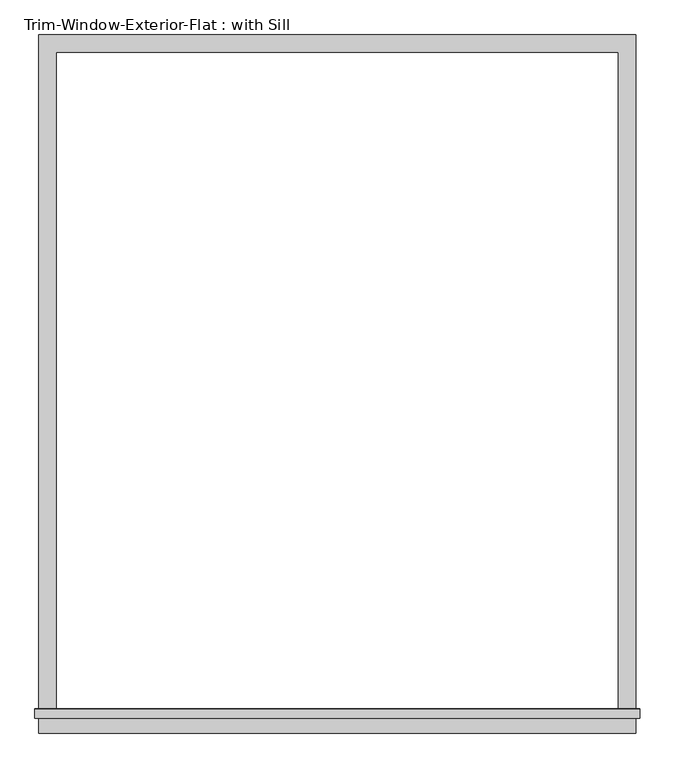
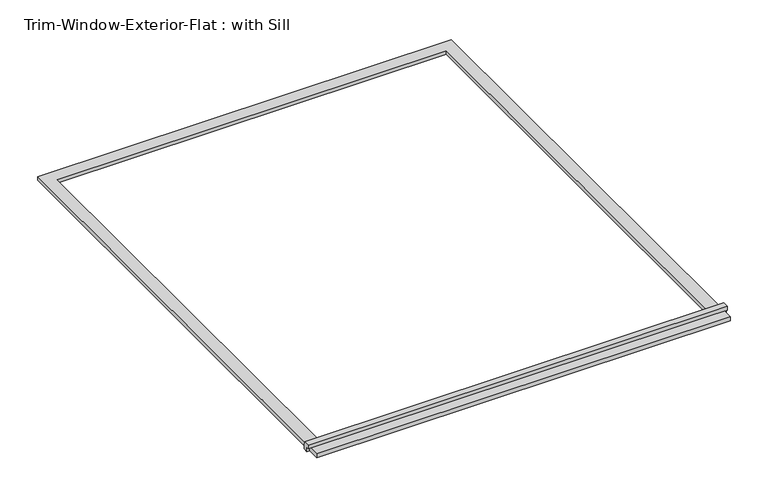
"""IFC4 building model written with IfcOpenShell, lengths in millimetres: proxy geometry, Trim-Window-Exterior-Flat : with Sill."""

from ifc_helpers import new_model, si_unit, frame, origin, origin_with_axes, place, context, project, spatial, polyline, outline, extrude, source, transform, mapped, element, save


def trim_window_exterior_flat_with_sill_384ab7b4(model_context):
    return source(origin(), model_context, "Body", "SweptSolid", [
        extrude(outline(polyline([(971.55, -2155.7823709), (971.55, -2212.9323709), (-971.55, -2212.9323709), (-971.55, -2155.7823709), (971.55, -2155.7823709)])), origin_with_axes(), (0.0, 0.0, 1.0), 19.05),
        extrude(outline(polyline([(-2165.35, 38.1), (-2136.0580645, 38.1), (-2133.6, 19.05), (-2133.6, 0.0), (-2155.7823709, 0.0), (-2155.7823709, 19.05), (-2165.35, 19.05), (-2165.35, 38.1)])), frame((-984.25, 0.0, 0.0), z_axis=(1.0, 0.0, 0.0), x_axis=(0.0, 1.0, 0.0)), (0.0, 0.0, 1.0), 1968.5),
        extrude(outline(polyline([(-971.55, 57.15), (971.55, 57.15), (971.55, -2133.6), (914.4, -2133.6), (914.4, 0.0), (-914.4, 0.0), (-914.4, -2133.6), (-971.55, -2133.6), (-971.55, 57.15)])), origin_with_axes(), (0.0, 0.0, 1.0), 19.05),
    ])


if __name__ == "__main__":
    model = new_model("IFC4")
    model_context = context("Model", 3, world=origin())
    ifc_project = project(units=[si_unit("LENGTHUNIT", "METRE", prefix="MILLI")], contexts=[model_context])
    site = spatial("IfcSite", under=ifc_project)
    building = spatial("IfcBuilding", under=site)
    placement = place(None, origin())
    trim_window_exterior_flat_with_sill_shape = trim_window_exterior_flat_with_sill_384ab7b4(model_context)
    element("IfcBuildingElementProxy", 1, Name="Trim-Window-Exterior-Flat : with Sill", ObjectType="Trim-Window-Exterior-Flat : with Sill", at=placement, inside=building, context=model_context, shape_type="MappedRepresentation", body=[
        mapped(trim_window_exterior_flat_with_sill_shape, transform((0.0, 0.0, 0.0), x_axis=(1.0, 0.0, 0.0), y_axis=(0.0, 1.0, 0.0), z_axis=(0.0, 0.0, 1.0))),
    ])
    save(model, "model.ifc")

# Revit data of these elements
# Type "Trim-Window-Exterior-Flat : with Sill"
#   Trim Width = 0' - 2 1/4"
#   Trim Thickness_Picture Frame = 0' - 1 1/4"
#   Trim Thickness_with Sill = 0' - 0 3/4"
#   Sill Thickness = 0' - 1 1/4"
#   Opening Width [instance default] = 2' - 0"
#   Opening Height [instance default] = 3' - 0"
#   Default Elevation = 4' - 0"
#   Sill = yes
#   Picture Frame = no
#   Trim Material [instance default] = none
# Element 1 (IfcBuildingElementProxy, "Trim-Window-Exterior-Flat : with Sill")
#   Opening Width = 6' - 0"
#   Opening Height = 7' - 0"
#   Trim Material = Clad - White
#   Materials on its faces: "Clad - White"
# Materials
#   "Clad - White": class "Wood", colour RGB 242 242 238, transparency 0, Cost = 0
